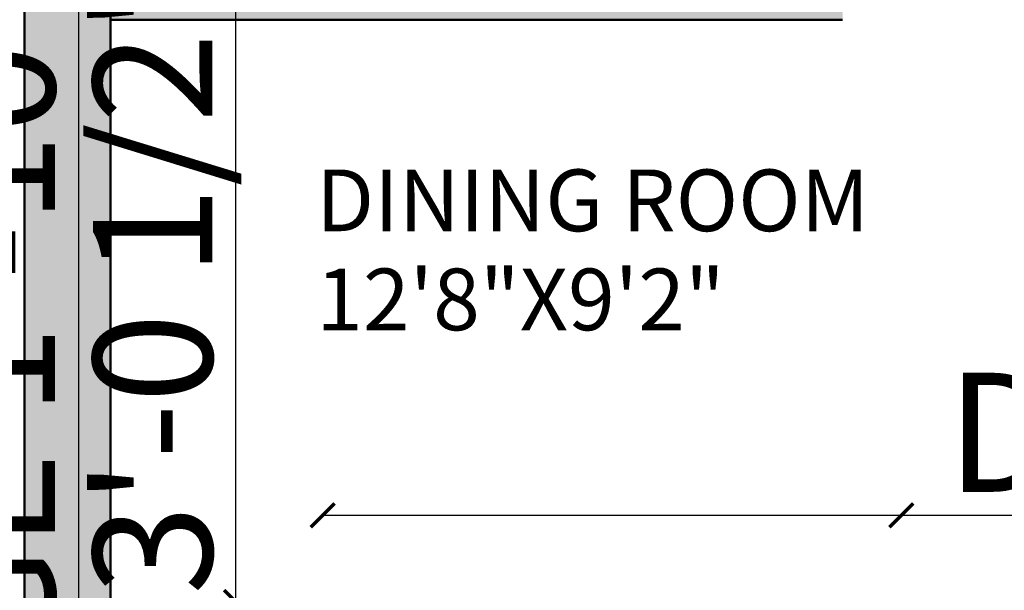
# Model space of a CAD drawing. Units: inches. Extents: x 2419 to 2878, y 1068 to 1713.
# Tile 7 of 20: x 2471 to 2574, y 1349 to 1409. Entities that reach past the tile are written whole.
import ezdxf

# ---------------------------------------------------------------- set-up
doc = ezdxf.new("R2010")
doc.units = ezdxf.units.IN
for name, color, linetype, lineweight in [('A-ANNO-DIMS', 2, 'Continuous', 18), ('A-AREA-IDEN', 7, 'Continuous', 18), ('A-FLOR-PRKG-PATT', 1, 'Continuous', 13), ('A-FURN-PATT', 254, 'Continuous', 13), ('A-WALL', 7, 'Continuous', 50)]:
    doc.layers.add(name, color=color, linetype=linetype, lineweight=lineweight)
doc.layers.add('A-FLOR-FIXT-PATT', color=254, linetype='Continuous', lineweight=13, true_color=0xd7ebd2)
doc.layers.add('A-WALL-PATT', color=18, linetype='Continuous', lineweight=13, true_color=0x000000)
doc.styles.get("Standard").update_dxf_attribs({"font": 'arial.ttf'})
doc.dimstyles.new('ISO-25', dxfattribs={"dimtxt": 12.5, "dimasz": 2.5, "dimexe": 1.25, "dimexo": 0.625, "dimtad": 1, "dimdec": 0, "dimlunit": 4, "dimtxsty": 'Standard', "dimblk": 'ARCHTICK', "dimcen": 2.5, "dimse1": 1, "dimse2": 1, "dimclrd": 4, "dimadec": 0, "dimazin": 0, "dimtfac": 1, "dimtdec": 0, "dimtmove": 0, "dimatfit": 3, "dimfxl": 1, "dimarcsym": 0})

# ---------------------------------------------------------------- blocks, each defined once
blk = doc.blocks.new('_ArchTick')
at = {"color": 0, "linetype": 'ByBlock', "const_width": 0.15}
blk.add_lwpolyline([(-0.5, -0.5), (0.5, 0.5)], dxfattribs=at)
blk = doc.blocks.new('*D26')
at = {"layer": 'A-ANNO-DIMS', "color": 4, "lineweight": -2, "transparency": 16777216}
for p, q in [((2502.77, 1356.79), (2563.46, 1356.79)), ((2563.46, 1356.79), (2733.72, 1356.79))]:
    blk.add_line(p, q, dxfattribs=at)
at = {"layer": 'Defpoints', "color": 0, "transparency": 16777216}
for p in [(2563.46, 1356.79), (2502.77, 1347.69), (2563.46, 1347.69)]:
    blk.add_point(p, dxfattribs=at)
at = {"layer": 'A-ANNO-DIMS', "color": 4, "lineweight": -2, "transparency": 16777216, "xscale": 2.5, "yscale": 2.5, "zscale": 2.5, "rotation": 180}
blk.add_blockref('_ArchTick', (2502.77, 1356.79), dxfattribs=at)
at = {"layer": 'A-ANNO-DIMS', "color": 4, "lineweight": -2, "transparency": 16777216, "xscale": 2.5, "yscale": 2.5, "zscale": 2.5}
blk.add_blockref('_ArchTick', (2563.46, 1356.79), dxfattribs=at)
at = {"layer": 'A-ANNO-DIMS', "color": 0, "transparency": 16777216, "insert": (2649.84, 1363.88), "char_height": 12.5, "attachment_point": 5}
blk.add_mtext('DINING SET 5\'-0 1/2"', dxfattribs=at)
blk = doc.blocks.new('*D27')
at = {"layer": 'A-ANNO-DIMS', "color": 4, "lineweight": -2, "transparency": 16777216}
for p, q in [((2493.67, 1347.69), (2493.67, 1413.78)), ((2493.67, 1311.01), (2493.67, 1347.69))]:
    blk.add_line(p, q, dxfattribs=at)
at = {"layer": 'Defpoints', "color": 0, "transparency": 16777216}
for p in [(2493.67, 1347.69), (2502.77, 1347.69), (2502.77, 1311.01)]:
    blk.add_point(p, dxfattribs=at)
at = {"layer": 'A-ANNO-DIMS', "color": 4, "lineweight": -2, "transparency": 16777216, "xscale": 2.5, "yscale": 2.5, "zscale": 2.5}
for p, rotation in [((2493.67, 1347.69), 90), ((2493.67, 1311.01), 270)]:
    blk.add_blockref('_ArchTick', p, dxfattribs=dict(at, rotation=rotation))
at = {"layer": 'A-ANNO-DIMS', "color": 0, "transparency": 16777216, "insert": (2486.57, 1381.99), "char_height": 12.5, "attachment_point": 5, "rotation": 90}
blk.add_mtext('3\'-0 1/2"', dxfattribs=at)
blk = doc.blocks.new('*D28')
at = {"layer": 'A-ANNO-DIMS', "color": 4, "lineweight": -2, "transparency": 16777216}
for p, q in [((2477.16, 1470.63), (2477.16, 1448.27)), ((2477.16, 1448.27), (2477.16, 1306.15))]:
    blk.add_line(p, q, dxfattribs=at)
at = {"layer": 'Defpoints', "color": 0, "transparency": 16777216}
for p in [(2480.51, 1470.63), (2477.16, 1448.27), (2480.51, 1448.27)]:
    blk.add_point(p, dxfattribs=at)
at = {"layer": 'A-ANNO-DIMS', "color": 4, "lineweight": -2, "transparency": 16777216, "xscale": 2.5, "yscale": 2.5, "zscale": 2.5}
for p, rotation in [((2477.16, 1470.63), 90), ((2477.16, 1448.27), 270)]:
    blk.add_blockref('_ArchTick', p, dxfattribs=dict(at, rotation=rotation))
at = {"layer": 'A-ANNO-DIMS', "color": 0, "transparency": 16777216, "insert": (2470.07, 1375.96), "char_height": 12.5, "attachment_point": 5, "rotation": 90}
blk.add_mtext('RANGE 1\'-10 1/2"', dxfattribs=at)
blk = doc.blocks.new('*D43')
at = {"layer": 'A-ANNO-DIMS', "color": 4, "lineweight": -2, "transparency": 16777216}
blk.add_line((2480.51, 1079.92), (2557.3, 1079.92), dxfattribs=at)
at = {"layer": 'Defpoints', "color": 0, "transparency": 16777216}
for p in [(2480.51, 1408.81), (2557.3, 1408.81), (2557.3, 1079.92)]:
    blk.add_point(p, dxfattribs=at)
at = {"layer": 'A-ANNO-DIMS', "color": 4, "lineweight": -2, "transparency": 16777216, "xscale": 2.5, "yscale": 2.5, "zscale": 2.5, "rotation": 180}
blk.add_blockref('_ArchTick', (2480.51, 1079.92), dxfattribs=at)
at = {"layer": 'A-ANNO-DIMS', "color": 4, "lineweight": -2, "transparency": 16777216, "xscale": 2.5, "yscale": 2.5, "zscale": 2.5}
blk.add_blockref('_ArchTick', (2557.3, 1079.92), dxfattribs=at)
at = {"layer": 'A-ANNO-DIMS', "color": 0, "transparency": 16777216, "insert": (2518.91, 1086.93), "char_height": 12.5, "attachment_point": 5}
blk.add_mtext('6\'-5"', dxfattribs=at)
blk = doc.blocks.new('*D44')
at = {"layer": 'A-ANNO-DIMS', "color": 4, "lineweight": -2, "transparency": 16777216}
for p, q in [((2557.3, 1079.92), (2585.82, 1079.92)), ((2585.82, 1079.92), (2652.14, 1079.92))]:
    blk.add_line(p, q, dxfattribs=at)
at = {"layer": 'Defpoints', "color": 0, "transparency": 16777216}
for p in [(2557.3, 1408.81), (2585.82, 1408.81), (2585.82, 1079.92)]:
    blk.add_point(p, dxfattribs=at)
at = {"layer": 'A-ANNO-DIMS', "color": 4, "lineweight": -2, "transparency": 16777216, "xscale": 2.5, "yscale": 2.5, "zscale": 2.5, "rotation": 180}
blk.add_blockref('_ArchTick', (2557.3, 1079.92), dxfattribs=at)
at = {"layer": 'A-ANNO-DIMS', "color": 4, "lineweight": -2, "transparency": 16777216, "xscale": 2.5, "yscale": 2.5, "zscale": 2.5}
blk.add_blockref('_ArchTick', (2585.82, 1079.92), dxfattribs=at)
at = {"layer": 'A-ANNO-DIMS', "color": 0, "transparency": 16777216, "insert": (2620.23, 1087.01), "char_height": 12.5, "attachment_point": 5}
blk.add_mtext('2\'-4 1/2"', dxfattribs=at)
blk = doc.blocks.new('*D47')
at = {"layer": 'A-ANNO-DIMS', "color": 4, "lineweight": -2, "transparency": 16777216}
for p, q in [((2444.31, 1376.56), (2444.31, 1357.98)), ((2444.31, 1357.98), (2444.31, 1293.05))]:
    blk.add_line(p, q, dxfattribs=at)
at = {"layer": 'Defpoints', "color": 0, "transparency": 16777216}
for p in [(2632.51, 1376.56), (2444.31, 1357.98), (2632.51, 1357.98)]:
    blk.add_point(p, dxfattribs=at)
at = {"layer": 'A-ANNO-DIMS', "color": 4, "lineweight": -2, "transparency": 16777216, "xscale": 2.5, "yscale": 2.5, "zscale": 2.5}
for p, rotation in [((2444.31, 1376.56), 90), ((2444.31, 1357.98), 270)]:
    blk.add_blockref('_ArchTick', p, dxfattribs=dict(at, rotation=rotation))
at = {"layer": 'A-ANNO-DIMS', "color": 0, "transparency": 16777216, "insert": (2437.23, 1324.26), "char_height": 12.5, "attachment_point": 5, "rotation": 90}
blk.add_mtext('1\'-6 1/2"', dxfattribs=at)
blk = doc.blocks.new('*D55')
at = {"layer": 'A-ANNO-DIMS', "color": 4, "lineweight": -2, "transparency": 16777216}
for p, q in [((2444.31, 1414.81), (2444.31, 1408.81)), ((2444.31, 1408.81), (2444.31, 1371.83))]:
    blk.add_line(p, q, dxfattribs=at)
at = {"layer": 'Defpoints', "color": 0, "transparency": 16777216}
for p in [(2480.51, 1414.81), (2444.31, 1408.81), (2480.51, 1408.81)]:
    blk.add_point(p, dxfattribs=at)
at = {"layer": 'A-ANNO-DIMS', "color": 4, "lineweight": -2, "transparency": 16777216, "xscale": 2.5, "yscale": 2.5, "zscale": 2.5}
for p, rotation in [((2444.31, 1414.81), 90), ((2444.31, 1408.81), 270)]:
    blk.add_blockref('_ArchTick', p, dxfattribs=dict(at, rotation=rotation))
at = {"layer": 'A-ANNO-DIMS', "color": 0, "transparency": 16777216, "insert": (2437.31, 1389.07), "char_height": 12.5, "attachment_point": 5, "rotation": 90}
blk.add_mtext('0\'-6"', dxfattribs=at)
blk = doc.blocks.new('*D56')
at = {"layer": 'A-ANNO-DIMS', "color": 4, "lineweight": -2, "transparency": 16777216}
for p, q in [((2480.51, 1079.92), (2503.97, 1079.92)), ((2503.97, 1079.92), (2578.61, 1079.92))]:
    blk.add_line(p, q, dxfattribs=at)
at = {"layer": 'Defpoints', "color": 0, "transparency": 16777216}
for p in [(2480.51, 1507.81), (2503.97, 1494.85), (2503.97, 1079.92)]:
    blk.add_point(p, dxfattribs=at)
at = {"layer": 'A-ANNO-DIMS', "color": 4, "lineweight": -2, "transparency": 16777216, "xscale": 2.5, "yscale": 2.5, "zscale": 2.5, "rotation": 180}
blk.add_blockref('_ArchTick', (2480.51, 1079.92), dxfattribs=at)
at = {"layer": 'A-ANNO-DIMS', "color": 4, "lineweight": -2, "transparency": 16777216, "xscale": 2.5, "yscale": 2.5, "zscale": 2.5}
blk.add_blockref('_ArchTick', (2503.97, 1079.92), dxfattribs=at)
at = {"layer": 'A-ANNO-DIMS', "color": 0, "transparency": 16777216, "insert": (2542.54, 1087.01), "char_height": 12.5, "attachment_point": 5}
blk.add_mtext('1\'-11 1/2"', dxfattribs=at)
blk = doc.blocks.new('*D59')
at = {"layer": 'A-ANNO-DIMS', "color": 4, "lineweight": -2, "transparency": 16777216}
blk.add_line((2480.51, 1079.92), (2589.51, 1079.92), dxfattribs=at)
at = {"layer": 'Defpoints', "color": 0, "transparency": 16777216}
for p in [(2480.51, 1414.81), (2589.51, 1414.81), (2589.51, 1079.92)]:
    blk.add_point(p, dxfattribs=at)
at = {"layer": 'A-ANNO-DIMS', "color": 4, "lineweight": -2, "transparency": 16777216, "xscale": 2.5, "yscale": 2.5, "zscale": 2.5, "rotation": 180}
blk.add_blockref('_ArchTick', (2480.51, 1079.92), dxfattribs=at)
at = {"layer": 'A-ANNO-DIMS', "color": 4, "lineweight": -2, "transparency": 16777216, "xscale": 2.5, "yscale": 2.5, "zscale": 2.5}
blk.add_blockref('_ArchTick', (2589.51, 1079.92), dxfattribs=at)
at = {"layer": 'A-ANNO-DIMS', "color": 0, "transparency": 16777216, "insert": (2535.01, 1086.93), "char_height": 12.5, "attachment_point": 5}
blk.add_mtext('9\'-1"', dxfattribs=at)

msp = doc.modelspace()

# ---------------------------------------------------------------- hatches: boundary and pattern name
at = {"layer": 'A-FLOR-FIXT-PATT'}
h = msp.add_hatch(color=256, dxfattribs=at)
h.dxf.hatch_style = 1
h.paths.add_polyline_path([(2771.51, 1458.39), (2763.51, 1458.39), (2763.51, 1437.39), (2771.51, 1437.39)])
h.paths.add_polyline_path([(2770.51, 1456.39, 0.5), (2769.51, 1457.39), (2765.51, 1457.39, 0.5), (2764.51, 1456.39), (2764.51, 1439.39, 0.5), (2765.51, 1438.39), (2769.51, 1438.39, 0.5), (2770.51, 1439.39)], flags=16)
h.paths.add_polyline_path([(2706.38, 1408.81), (2685.38, 1408.81), (2685.38, 1400.81), (2706.38, 1400.81)])
h.paths.add_polyline_path([(2704.38, 1401.81, 0.5), (2705.38, 1402.81), (2705.38, 1406.81, 0.5), (2704.38, 1407.81), (2687.38, 1407.81, 0.5), (2686.38, 1406.81), (2686.38, 1402.81, 0.5), (2687.38, 1401.81)], flags=16)
h.paths.add_polyline_path([(2574.48, 1207.45), (2633.94, 1207.45), (2633.94, 1217.37), (2574.48, 1217.37)], flags=9)
h.paths.add_polyline_path([(2574.45, 1217.83), (2610.47, 1217.83), (2610.47, 1227.88), (2574.45, 1227.88)], flags=9)
h.paths.add_polyline_path([(2672.43, 1304.02), (2718.62, 1304.02), (2718.62, 1313.94), (2672.43, 1313.94)], flags=9)
h.paths.add_polyline_path([(2672.4, 1314.4), (2750.13, 1314.4), (2750.13, 1324.45), (2672.4, 1324.45)], flags=9)
h.paths.add_polyline_path([(2500.43, 1374.44), (2544.8, 1374.44), (2544.8, 1384.36), (2500.43, 1384.36)], flags=9)
h.paths.add_polyline_path([(2500.41, 1384.82), (2566.08, 1384.82), (2566.08, 1394.87), (2500.41, 1394.87)], flags=9)
h.paths.add_polyline_path([(2738.93, 1376.75), (2778.27, 1376.75), (2778.27, 1386.67), (2738.93, 1386.67)], flags=9)
h.paths.add_polyline_path([(2659.12, 1357.8), (2703.49, 1357.8), (2703.49, 1367.72), (2659.12, 1367.72)], flags=9)
h.paths.add_polyline_path([(2659.1, 1368.18), (2694.11, 1368.18), (2694.11, 1378.23), (2659.1, 1378.23)], flags=9)
h.paths.add_polyline_path([(2730.12, 1466.07), (2769.46, 1466.07), (2769.46, 1475.99), (2730.12, 1475.99)], flags=9)
h.paths.add_polyline_path([(2730.1, 1476.45), (2765.12, 1476.45), (2765.12, 1486.5), (2730.1, 1486.5)], flags=9)
h.paths.add_polyline_path([(2730.38, 1518.65), (2761.48, 1518.65), (2761.48, 1528.57), (2730.38, 1528.57)], flags=9)
h.paths.add_polyline_path([(2730.36, 1529.03), (2780.96, 1529.03), (2780.96, 1539.07), (2730.36, 1539.07)], flags=9)
h.paths.add_polyline_path([(2629.32, 1455.19), (2688.78, 1455.19), (2688.78, 1465.11), (2629.32, 1465.11)], flags=9)
h.paths.add_polyline_path([(2629.3, 1465.57), (2681.9, 1465.57), (2681.9, 1475.62), (2629.3, 1475.62)], flags=9)
h.paths.add_polyline_path([(2513.23, 1456.48), (2562.63, 1456.48), (2562.63, 1466.4), (2513.23, 1466.4)], flags=9)
h.paths.add_polyline_path([(2513.21, 1466.86), (2556.26, 1466.86), (2556.26, 1476.91), (2513.21, 1476.91)], flags=9)
h.paths.add_polyline_path([(2488.87, 1521.54), (2519.97, 1521.54), (2519.97, 1531.46), (2488.87, 1531.46)], flags=9)
h.paths.add_polyline_path([(2536.55, 1543.51), (2580.92, 1543.51), (2580.92, 1553.43), (2536.55, 1553.43)], flags=9)
h.paths.add_polyline_path([(2536.56, 1553.92), (2573.53, 1553.92), (2573.53, 1563.8), (2536.56, 1563.8)], flags=9)
at = {"layer": 'A-FLOR-PRKG-PATT'}
h = msp.add_hatch(color=256, dxfattribs=at)
h.dxf.hatch_style = 1
edge = h.paths.add_edge_path()
edge.add_ellipse((2561.37, 1279.45), major_axis=(3.99, 0), ratio=0.842304, start_angle=0.6466, end_angle=90)
edge.add_line((2561.37, 1282.81), (2511.57, 1282.81))
edge.add_ellipse((2511.57, 1279.45), major_axis=(3.99, 0), ratio=0.842304, start_angle=90, end_angle=179.3534)
edge.add_ellipse((10560.89, 1188.62), major_axis=(-8054.03, 0), ratio=0.8423039, start_angle=-0.646554, end_angle=-0.628237)
edge.add_ellipse((2509.23, 1276.91), major_axis=(1.69, 0), ratio=0.842304, start_angle=179.3718, end_angle=248.4648)
edge.add_ellipse((10560.33, 1188.62), major_axis=(8052.29, 0), ratio=0.8423039, start_angle=179.353446, end_angle=179.381357, ccw=False)
edge.add_ellipse((2511.01, 1279.45), major_axis=(2.25, 0), ratio=0.842304, start_angle=90, end_angle=179.3534, ccw=False)
edge.add_line((2511.01, 1281.35), (2561.94, 1281.35))
edge.add_ellipse((2561.94, 1279.45), major_axis=(-2.25, 0), ratio=0.842304, start_angle=180.6466, end_angle=270, ccw=False)
edge.add_ellipse((-5487.38, 1188.62), major_axis=(8052.29, 0), ratio=0.8423039, start_angle=0.528271, end_angle=0.646554, ccw=False)
edge.add_ellipse((2563.71, 1276.91), major_axis=(-1.69, 0), ratio=0.842304, start_angle=111.5352, end_angle=180.6282)
edge.add_ellipse((-5487.95, 1188.62), major_axis=(-8054.03, 0), ratio=0.8423039, start_angle=180.628237, end_angle=180.646554)
edge = h.paths.add_edge_path()
edge.add_ellipse((2564.91, 1261.91), major_axis=(-1.12, 0), ratio=0.842304, start_angle=180, end_angle=270)
edge.add_line((2564.91, 1262.86), (2564.43, 1262.86))
edge.add_ellipse((-5487.38, 1188.62), major_axis=(8052.29, 0), ratio=0.8423039, start_angle=0.383867, end_angle=0.528271, ccw=False)
edge.add_line((2564.65, 1242.56), (2564.91, 1242.56))
edge.add_ellipse((2564.91, 1243.51), major_axis=(-1.12, 0), ratio=0.842304, start_angle=90, end_angle=180)
edge.add_line((2566.03, 1243.51), (2566.03, 1261.91))
edge = h.paths.add_edge_path()
edge.add_ellipse((2564.91, 1174.99), major_axis=(1.12, 0), ratio=0.842304, start_angle=0, end_angle=90)
edge.add_line((2564.91, 1175.94), (2564.89, 1175.94))
edge.add_ellipse((-5487.38, 1188.62), major_axis=(8052.29, 0), ratio=0.8423039, start_angle=-0.134987, end_angle=-0.090229, ccw=False)
edge.add_ellipse((2163.34, 1170.91), major_axis=(401.54, 0), ratio=0.842304, start_angle=-2.18, end_angle=-0.1356, ccw=False)
edge.add_line((2564.47, 1155.64), (2564.91, 1155.64))
edge.add_ellipse((2564.91, 1156.59), major_axis=(-1.12, 0), ratio=0.842304, start_angle=90, end_angle=180)
edge.add_line((2566.03, 1156.59), (2566.03, 1174.99))
h.paths.add_polyline_path([(2574.48, 1207.45), (2633.94, 1207.45), (2633.94, 1217.37), (2574.48, 1217.37)], flags=9)
h.paths.add_polyline_path([(2574.45, 1217.83), (2610.47, 1217.83), (2610.47, 1227.88), (2574.45, 1227.88)], flags=9)
h.paths.add_polyline_path([(2672.43, 1304.02), (2718.62, 1304.02), (2718.62, 1313.94), (2672.43, 1313.94)], flags=9)
h.paths.add_polyline_path([(2672.4, 1314.4), (2750.13, 1314.4), (2750.13, 1324.45), (2672.4, 1324.45)], flags=9)
h.paths.add_polyline_path([(2500.43, 1374.44), (2544.8, 1374.44), (2544.8, 1384.36), (2500.43, 1384.36)], flags=9)
h.paths.add_polyline_path([(2500.41, 1384.82), (2566.08, 1384.82), (2566.08, 1394.87), (2500.41, 1394.87)], flags=9)
h.paths.add_polyline_path([(2738.93, 1376.75), (2778.27, 1376.75), (2778.27, 1386.67), (2738.93, 1386.67)], flags=9)
h.paths.add_polyline_path([(2659.12, 1357.8), (2703.49, 1357.8), (2703.49, 1367.72), (2659.12, 1367.72)], flags=9)
h.paths.add_polyline_path([(2659.1, 1368.18), (2694.11, 1368.18), (2694.11, 1378.23), (2659.1, 1378.23)], flags=9)
h.paths.add_polyline_path([(2730.12, 1466.07), (2769.46, 1466.07), (2769.46, 1475.99), (2730.12, 1475.99)], flags=9)
h.paths.add_polyline_path([(2730.1, 1476.45), (2765.12, 1476.45), (2765.12, 1486.5), (2730.1, 1486.5)], flags=9)
h.paths.add_polyline_path([(2730.38, 1518.65), (2761.48, 1518.65), (2761.48, 1528.57), (2730.38, 1528.57)], flags=9)
h.paths.add_polyline_path([(2730.36, 1529.03), (2780.96, 1529.03), (2780.96, 1539.07), (2730.36, 1539.07)], flags=9)
h.paths.add_polyline_path([(2629.32, 1455.19), (2688.78, 1455.19), (2688.78, 1465.11), (2629.32, 1465.11)], flags=9)
h.paths.add_polyline_path([(2629.3, 1465.57), (2681.9, 1465.57), (2681.9, 1475.62), (2629.3, 1475.62)], flags=9)
h.paths.add_polyline_path([(2513.23, 1456.48), (2562.63, 1456.48), (2562.63, 1466.4), (2513.23, 1466.4)], flags=9)
h.paths.add_polyline_path([(2513.21, 1466.86), (2556.26, 1466.86), (2556.26, 1476.91), (2513.21, 1476.91)], flags=9)
h.paths.add_polyline_path([(2488.87, 1521.54), (2519.97, 1521.54), (2519.97, 1531.46), (2488.87, 1531.46)], flags=9)
h.paths.add_polyline_path([(2536.55, 1543.51), (2580.92, 1543.51), (2580.92, 1553.43), (2536.55, 1553.43)], flags=9)
h.paths.add_polyline_path([(2536.56, 1553.92), (2573.53, 1553.92), (2573.53, 1563.8), (2536.56, 1563.8)], flags=9)
at = {"layer": 'A-FURN-PATT'}
h = msp.add_hatch(color=256, dxfattribs=at)
h.dxf.hatch_style = 1
h.paths.add_polyline_path([(2710.17, 1562.64), (2707.17, 1559.64), (2709.17, 1559.64, -0.414214), (2710.17, 1560.64)])
h.paths.add_polyline_path([(2711.17, 1559.64, 1), (2709.17, 1559.64, 1)])
h.paths.add_polyline_path([(2710.17, 1562.64), (2710.17, 1560.64, -0.414214), (2711.17, 1559.64), (2713.17, 1559.64)])
h.paths.add_polyline_path([(2713.17, 1559.64), (2711.17, 1559.64, -0.414214), (2710.17, 1558.64), (2710.17, 1556.64)])
h.paths.add_polyline_path([(2710.17, 1558.64, -0.414214), (2709.17, 1559.64), (2707.17, 1559.64), (2710.17, 1556.64)])
h.paths.add_polyline_path([(2613.13, 1558.89, 1), (2611.13, 1558.89, 1)])
h.paths.add_polyline_path([(2612.13, 1561.89), (2612.13, 1559.89, -0.414214), (2613.13, 1558.89), (2615.13, 1558.89)])
h.paths.add_polyline_path([(2612.13, 1559.89), (2612.13, 1561.89), (2609.13, 1558.89), (2611.13, 1558.89, -0.414214)])
h.paths.add_polyline_path([(2612.13, 1557.89, -0.414214), (2611.13, 1558.89), (2609.13, 1558.89), (2612.13, 1555.89)])
h.paths.add_polyline_path([(2574.48, 1207.45), (2633.94, 1207.45), (2633.94, 1217.37), (2574.48, 1217.37)], flags=9)
h.paths.add_polyline_path([(2574.45, 1217.83), (2610.47, 1217.83), (2610.47, 1227.88), (2574.45, 1227.88)], flags=9)
h.paths.add_polyline_path([(2672.43, 1304.02), (2718.62, 1304.02), (2718.62, 1313.94), (2672.43, 1313.94)], flags=9)
h.paths.add_polyline_path([(2672.4, 1314.4), (2750.13, 1314.4), (2750.13, 1324.45), (2672.4, 1324.45)], flags=9)
h.paths.add_polyline_path([(2500.43, 1374.44), (2544.8, 1374.44), (2544.8, 1384.36), (2500.43, 1384.36)], flags=9)
h.paths.add_polyline_path([(2500.41, 1384.82), (2566.08, 1384.82), (2566.08, 1394.87), (2500.41, 1394.87)], flags=9)
h.paths.add_polyline_path([(2738.93, 1376.75), (2778.27, 1376.75), (2778.27, 1386.67), (2738.93, 1386.67)], flags=9)
h.paths.add_polyline_path([(2659.12, 1357.8), (2703.49, 1357.8), (2703.49, 1367.72), (2659.12, 1367.72)], flags=9)
h.paths.add_polyline_path([(2659.1, 1368.18), (2694.11, 1368.18), (2694.11, 1378.23), (2659.1, 1378.23)], flags=9)
h.paths.add_polyline_path([(2730.12, 1466.07), (2769.46, 1466.07), (2769.46, 1475.99), (2730.12, 1475.99)], flags=9)
h.paths.add_polyline_path([(2730.1, 1476.45), (2765.12, 1476.45), (2765.12, 1486.5), (2730.1, 1486.5)], flags=9)
h.paths.add_polyline_path([(2730.38, 1518.65), (2761.48, 1518.65), (2761.48, 1528.57), (2730.38, 1528.57)], flags=9)
h.paths.add_polyline_path([(2730.36, 1529.03), (2780.96, 1529.03), (2780.96, 1539.07), (2730.36, 1539.07)], flags=9)
h.paths.add_polyline_path([(2629.32, 1455.19), (2688.78, 1455.19), (2688.78, 1465.11), (2629.32, 1465.11)], flags=9)
h.paths.add_polyline_path([(2629.3, 1465.57), (2681.9, 1465.57), (2681.9, 1475.62), (2629.3, 1475.62)], flags=9)
h.paths.add_polyline_path([(2513.23, 1456.48), (2562.63, 1456.48), (2562.63, 1466.4), (2513.23, 1466.4)], flags=9)
h.paths.add_polyline_path([(2513.21, 1466.86), (2556.26, 1466.86), (2556.26, 1476.91), (2513.21, 1476.91)], flags=9)
h.paths.add_polyline_path([(2488.87, 1521.54), (2519.97, 1521.54), (2519.97, 1531.46), (2488.87, 1531.46)], flags=9)
h.paths.add_polyline_path([(2536.55, 1543.51), (2580.92, 1543.51), (2580.92, 1553.43), (2536.55, 1553.43)], flags=9)
h.paths.add_polyline_path([(2536.56, 1553.92), (2573.53, 1553.92), (2573.53, 1563.8), (2536.56, 1563.8)], flags=9)
at = {"layer": 'A-WALL-PATT'}
h = msp.add_hatch(color=256, dxfattribs=at)
h.dxf.hatch_style = 1
h.paths.add_polyline_path([(2780.51, 1577.81), (2471.51, 1577.81), (2471.51, 1121.81), (2780.51, 1121.81)])
h.paths.add_polyline_path([(2480.51, 1568.81), (2771.51, 1568.81), (2771.51, 1130.81), (2480.51, 1130.81)], flags=16)
h.paths.add_polyline_path([(2528.51, 1568.81), (2528.51, 1512.81), (2594.51, 1512.81), (2594.51, 1414.81), (2596.57, 1414.81), (2596.57, 1441.61), (2597.82, 1441.61), (2597.82, 1441.58, -0.384016), (2625.03, 1414.81), (2725.51, 1414.81), (2725.51, 1567.55), (2728.3, 1567.55), (2746.89, 1567.55), (2746.89, 1566.73), (2746.87, 1566.73, -0.367216), (2730.51, 1549.09), (2730.51, 1512.81), (2750.85, 1512.81), (2750.85, 1510.03, -0.401453), (2733.08, 1491.46), (2733.08, 1491.44), (2732.27, 1491.44), (2732.27, 1507.81), (2730.51, 1507.81), (2730.51, 1408.81), (2736.51, 1408.81), (2736.51, 1349.81), (2632.51, 1349.81), (2632.51, 1408.81), (2528.51, 1408.81), (2528.51, 1414.81), (2503.97, 1414.81), (2503.97, 1494.85), (2558.38, 1494.85), (2558.38, 1507.81), (2529.96, 1507.81, -0.414214), (2530.82, 1506.96), (2530.82, 1497.26, -0.414214), (2529.96, 1496.4), (2514.56, 1496.4, -0.414214), (2513.7, 1497.26), (2513.7, 1506.96, -0.414214), (2514.56, 1507.81), (2528.51, 1507.81), (2528.51, 1512.81), (2480.51, 1512.81)], flags=0)
h.paths.add_polyline_path([(2516.26, 1507.81), (2528.26, 1507.81), (2528.26, 1505.81), (2523.42, 1505.81), (2524.07, 1504.67), (2529.39, 1504.67, -0.414214), (2529.96, 1504.1), (2529.96, 1497.83, -0.414214), (2529.39, 1497.26), (2515.13, 1497.26, -0.414214), (2514.56, 1497.83), (2514.56, 1504.1, -0.414214), (2515.13, 1504.67), (2520.69, 1504.67), (2521.34, 1505.81), (2516.26, 1505.81)], flags=0)
h.paths.add_polyline_path([(2522.02, 1505.53), (2522.82, 1507.32, -0.65506), (2522.25, 1506.06), (2522.19, 1505.93), (2522.43, 1505.53)], flags=0)
h.paths.add_polyline_path([(2522.83, 1500.97, -1), (2521.69, 1500.97, -1)], flags=0)
h.paths.add_polyline_path([(2522.55, 1500.97, -1), (2521.98, 1500.97, -1)], flags=0)
h.paths.add_polyline_path([(2482.01, 1470.63), (2499.89, 1470.63), (2499.89, 1448.27), (2482.01, 1448.27), (2482.01, 1452.74), (2481.26, 1452.74), (2481.26, 1449.76), (2480.51, 1449.76), (2480.51, 1469.14), (2481.26, 1469.14), (2481.26, 1466.16), (2482.01, 1466.16)], flags=0)
h.paths.add_polyline_path([(2488.71, 1466.16, -1), (2484.24, 1466.16, -1)], flags=0)
h.paths.add_polyline_path([(2496.17, 1466.16, -1), (2490.2, 1466.16, -1)], flags=0)
h.paths.add_polyline_path([(2487.97, 1466.16, -1), (2484.99, 1466.16, -1)], flags=0)
h.paths.add_polyline_path([(2495.42, 1466.16, -1), (2490.95, 1466.16, -1)], flags=0)
h.paths.add_polyline_path([(2487.22, 1466.16, -1), (2485.73, 1466.16, -1)], flags=0)
h.paths.add_polyline_path([(2494.68, 1466.16, -1), (2491.69, 1466.16, -1)], flags=0)
h.paths.add_polyline_path([(2499.11, 1468, -1), (2497.98, 1468, -1)], flags=0)
h.paths.add_polyline_path([(2493.93, 1466.16, -1), (2492.44, 1466.16, -1)], flags=0)
h.paths.add_polyline_path([(2499.37, 1463.71, -1), (2498.17, 1463.71, -1)], flags=0)
h.paths.add_polyline_path([(2484.24, 1461.69), (2496.17, 1461.69), (2496.17, 1457.22), (2484.24, 1457.22)], flags=0)
h.paths.add_polyline_path([(2484.99, 1460.94), (2495.42, 1460.94), (2495.42, 1457.96), (2484.99, 1457.96)], flags=0)
h.paths.add_polyline_path([(2586.88, 1510.03), (2587.69, 1510.03), (2587.69, 1491.44), (2586.88, 1491.44)], flags=0)
h.paths.add_polyline_path([(2499.26, 1459.41, -1), (2498.2, 1459.41, -1)], flags=0)
h.paths.add_polyline_path([(2489.46, 1452.74, -1), (2483.5, 1452.74, -1)], flags=0)
h.paths.add_polyline_path([(2557.3, 1408.81), (2557.3, 1413.09, -0.401453), (2584.57, 1441.58), (2584.57, 1441.61), (2585.82, 1441.61), (2585.82, 1413.09), (2585.82, 1408.81)], flags=0)
h.paths.add_polyline_path([(2488.71, 1452.74, -1), (2484.24, 1452.74, -1)], flags=0)
h.paths.add_polyline_path([(2495.42, 1452.74, -1), (2490.95, 1452.74, -1)], flags=0)
h.paths.add_polyline_path([(2487.97, 1452.74, -1), (2484.99, 1452.74, -1)], flags=0)
h.paths.add_polyline_path([(2494.68, 1452.74, -1), (2491.69, 1452.74, -1)], flags=0)
h.paths.add_polyline_path([(2487.22, 1452.74, -1), (2485.73, 1452.74, -1)], flags=0)
h.paths.add_polyline_path([(2499.18, 1454.44, -1), (2497.9, 1454.44, -1)], flags=0)
h.paths.add_polyline_path([(2493.93, 1452.74, -1), (2492.44, 1452.74, -1)], flags=0)
h.paths.add_polyline_path([(2499.3, 1450.64, -1), (2497.79, 1450.64, -1)], flags=0)
h.paths.add_polyline_path([(2619.13, 1558.89, -1), (2605.13, 1558.89, -1)], flags=0)
h.paths.add_polyline_path([(2609.13, 1558.89), (2612.13, 1561.89), (2615.13, 1558.89), (2612.13, 1555.89)], flags=0)
h.paths.add_polyline_path([(2611.13, 1558.89, -1), (2613.13, 1558.89, -1)], flags=0)
h.paths.add_polyline_path([(2633.68, 1568.81), (2693.68, 1568.81), (2693.68, 1488.81), (2633.68, 1488.81)], flags=0)
h.paths.add_polyline_path([(2641.68, 1554.41), (2641.68, 1567.61), (2662.48, 1567.61), (2662.48, 1554.41), (2664.88, 1554.41), (2664.88, 1567.61), (2685.68, 1567.61), (2685.68, 1552.41), (2680.48, 1552.41), (2693.68, 1539.21), (2678.48, 1539.21), (2678.48, 1554.41)], flags=0)
h.paths.add_polyline_path([(2637.51, 1408.81), (2731.51, 1408.81), (2731.51, 1354.81), (2637.51, 1354.81), (2637.51, 1357.98), (2635.3, 1357.98), (2635.3, 1358.79), (2637.51, 1358.79)], flags=0)
h.paths.add_polyline_path([(2717.17, 1559.64, -1), (2703.17, 1559.64, -1)], flags=0)
h.paths.add_polyline_path([(2707.17, 1559.64), (2710.17, 1562.64), (2713.17, 1559.64), (2710.17, 1556.64)], flags=0)
h.paths.add_polyline_path([(2709.17, 1559.64, -1), (2711.17, 1559.64, -1)], flags=0)
h.paths.add_polyline_path([(2685.38, 1408.81), (2706.38, 1408.81), (2706.38, 1400.81), (2699.88, 1400.81), (2701.88, 1394.81, -0.501323), (2696.92, 1375.95, -0.132891), (2694.83, 1375.95, -0.501317), (2689.88, 1394.81), (2691.88, 1400.81), (2688.88, 1400.81), (2688.88, 1399.31), (2685.88, 1399.31), (2685.88, 1400.31), (2687.88, 1400.31), (2687.88, 1400.81), (2685.38, 1400.81)], flags=0)
h.paths.add_polyline_path([(2687.38, 1407.81), (2704.38, 1407.81, -0.5), (2705.38, 1406.81), (2705.38, 1402.81, -0.5), (2704.38, 1401.81), (2687.38, 1401.81, -0.5), (2686.38, 1402.81), (2686.38, 1406.81, -0.5)], flags=0)
h.paths.add_polyline_path([(2639.51, 1205.81), (2634.51, 1205.81), (2634.51, 1293.81), (2637.51, 1293.81), (2639.51, 1293.81)], flags=0)
h.paths.add_polyline_path([(2691.88, 1394.81), (2699.88, 1394.81, -0.48008), (2697.52, 1377.29, -0.215004), (2694.23, 1377.29, -0.48008)], flags=0)
h.paths.add_polyline_path([(2757.51, 1453.89), (2763.51, 1451.89), (2763.51, 1454.89), (2762.01, 1454.89), (2762.01, 1457.89), (2763.01, 1457.89), (2763.01, 1455.89), (2763.51, 1455.89), (2763.51, 1458.39), (2771.51, 1458.39), (2771.51, 1437.39), (2763.51, 1437.39), (2763.51, 1443.89), (2757.51, 1441.89, -0.501323), (2738.65, 1446.85, -0.132891), (2738.65, 1448.94, -0.501317)], flags=0)
h.paths.add_polyline_path([(2739.99, 1449.54, -0.48008), (2757.51, 1451.89), (2757.51, 1443.89, -0.48008), (2739.99, 1446.25, -0.215004)], flags=0)
h.paths.add_polyline_path([(2765.51, 1457.39), (2769.51, 1457.39, -0.5), (2770.51, 1456.39), (2770.51, 1439.39, -0.5), (2769.51, 1438.39), (2765.51, 1438.39, -0.5), (2764.51, 1439.39), (2764.51, 1456.39, -0.5)], flags=0)
h = msp.add_hatch(color=256, dxfattribs=at)
h.dxf.hatch_style = 1
h.paths.add_polyline_path([(2771.51, 1354.81), (2736.51, 1354.81), (2736.51, 1408.81), (2771.51, 1408.81), (2771.51, 1414.81), (2625.03, 1414.81, -0.015108), (2625.09, 1413.09), (2625.09, 1408.81), (2632.51, 1408.81), (2632.51, 1376.56), (2635.3, 1376.56, -0.029838), (2637.51, 1376.43), (2637.51, 1408.81), (2731.51, 1408.81), (2731.51, 1354.81), (2637.51, 1354.81), (2637.51, 1357.98), (2635.3, 1357.98), (2632.51, 1357.98), (2632.51, 1349.81), (2771.51, 1349.81)])
h.paths.add_polyline_path([(2639.51, 1298.81), (2637.51, 1298.81), (2480.51, 1298.81), (2480.51, 1293.81), (2637.51, 1293.81), (2639.51, 1293.81)])
h.paths.add_polyline_path([(2639.51, 1293.81), (2637.51, 1293.81), (2634.51, 1293.81), (2634.51, 1244.65), (2638.79, 1244.65, -0.006332), (2639.51, 1244.64)])
h.paths.add_polyline_path([(2639.51, 1205.81), (2771.51, 1205.81), (2771.51, 1210.81), (2639.51, 1210.81), (2639.51, 1216.13), (2638.79, 1216.13), (2634.51, 1216.13), (2634.51, 1130.81), (2639.51, 1130.81)])
h.paths.add_polyline_path([(2596.57, 1413.09), (2596.57, 1414.81), (2585.82, 1414.81), (2585.82, 1413.09), (2585.82, 1408.81), (2596.57, 1408.81)])
h.paths.add_polyline_path([(2557.3, 1413.09, -0.015108), (2557.35, 1414.81), (2480.51, 1414.81), (2480.51, 1408.81), (2557.3, 1408.81)])
h.paths.add_polyline_path([(2574.48, 1207.45), (2633.94, 1207.45), (2633.94, 1217.37), (2574.48, 1217.37)], flags=9)
h.paths.add_polyline_path([(2574.45, 1217.83), (2610.47, 1217.83), (2610.47, 1227.88), (2574.45, 1227.88)], flags=9)
h.paths.add_polyline_path([(2672.43, 1304.02), (2718.62, 1304.02), (2718.62, 1313.94), (2672.43, 1313.94)], flags=9)
h.paths.add_polyline_path([(2672.4, 1314.4), (2750.13, 1314.4), (2750.13, 1324.45), (2672.4, 1324.45)], flags=9)
h.paths.add_polyline_path([(2500.43, 1374.44), (2544.8, 1374.44), (2544.8, 1384.36), (2500.43, 1384.36)], flags=9)
h.paths.add_polyline_path([(2500.41, 1384.82), (2566.08, 1384.82), (2566.08, 1394.87), (2500.41, 1394.87)], flags=9)
h.paths.add_polyline_path([(2738.93, 1376.75), (2778.27, 1376.75), (2778.27, 1386.67), (2738.93, 1386.67)], flags=9)
h.paths.add_polyline_path([(2659.12, 1357.8), (2703.49, 1357.8), (2703.49, 1367.72), (2659.12, 1367.72)], flags=25)
h.paths.add_polyline_path([(2659.1, 1368.18), (2694.11, 1368.18), (2694.11, 1378.23), (2659.1, 1378.23)], flags=25)
h.paths.add_polyline_path([(2730.12, 1466.07), (2769.46, 1466.07), (2769.46, 1475.99), (2730.12, 1475.99)], flags=9)
h.paths.add_polyline_path([(2730.1, 1476.45), (2765.12, 1476.45), (2765.12, 1486.5), (2730.1, 1486.5)], flags=9)
h.paths.add_polyline_path([(2730.38, 1518.65), (2761.48, 1518.65), (2761.48, 1528.57), (2730.38, 1528.57)], flags=9)
h.paths.add_polyline_path([(2730.36, 1529.03), (2780.96, 1529.03), (2780.96, 1539.07), (2730.36, 1539.07)], flags=9)
h.paths.add_polyline_path([(2629.32, 1455.19), (2688.78, 1455.19), (2688.78, 1465.11), (2629.32, 1465.11)], flags=9)
h.paths.add_polyline_path([(2629.3, 1465.57), (2681.9, 1465.57), (2681.9, 1475.62), (2629.3, 1475.62)], flags=9)
h.paths.add_polyline_path([(2513.23, 1456.48), (2562.63, 1456.48), (2562.63, 1466.4), (2513.23, 1466.4)], flags=9)
h.paths.add_polyline_path([(2513.21, 1466.86), (2556.26, 1466.86), (2556.26, 1476.91), (2513.21, 1476.91)], flags=9)
h.paths.add_polyline_path([(2488.87, 1521.54), (2519.97, 1521.54), (2519.97, 1531.46), (2488.87, 1531.46)], flags=9)
h.paths.add_polyline_path([(2536.55, 1543.51), (2580.92, 1543.51), (2580.92, 1553.43), (2536.55, 1553.43)], flags=9)
h.paths.add_polyline_path([(2536.56, 1553.92), (2573.53, 1553.92), (2573.53, 1563.8), (2536.56, 1563.8)], flags=9)

# ---------------------------------------------------------------- linework, layer by layer
at = {"layer": 'A-WALL'}
for p, q in [((2480.51, 1130.81), (2480.51, 1568.81)), ((2480.51, 1408.81), (2557.3, 1408.81)), ((2480.51, 1408.81), (2557.3, 1408.81))]:
    msp.add_line(p, q, dxfattribs=at)
msp.add_lwpolyline([(2471.51, 1577.81), (2780.51, 1577.81), (2780.51, 1121.81), (2471.51, 1121.81)], close=True, dxfattribs=at)

# ---------------------------------------------------------------- texts
at = {"layer": 'A-AREA-IDEN'}
for s, height, p in [('DINING ROOM', 6.4753, (2502.09, 1386.61)), ('12\'8"X9\'2"', 6.475, (2502.09, 1376.21))]:
    msp.add_text(s, height=height, dxfattribs=at).set_placement(p)

# ---------------------------------------------------------------- dimensions: what is measured, and where the dimension line sits
at = {"layer": 'A-ANNO-DIMS'}
for base, p1, p2, picture, middle in [((2503.97, 1079.92), (2480.51, 1507.81), (2503.97, 1494.85), '*D56', (2542.54, 1087.01)), ((2589.51, 1079.92), (2480.51, 1414.81), (2589.51, 1414.81), '*D59', (2535.01, 1086.93)), ((2557.3, 1079.92), (2480.51, 1408.81), (2557.3, 1408.81), '*D43', (2518.91, 1086.93)), ((2585.82, 1079.92), (2557.3, 1408.81), (2585.82, 1408.81), '*D44', (2620.23, 1087.01))]:
    dim = msp.add_linear_dim(base=base, p1=p1, p2=p2, dimstyle='ISO-25', override={"dimdec": 1, "dimlfac": 1, "dimrnd": 0, "dimzin": 1, "dimdsep": 46, "dimlunit": 4, "dimfrac": 2}, dxfattribs=at)
    dim.commit()
    dim.dimension.update_dxf_attribs({"geometry": picture, "text_midpoint": middle})
dim = msp.add_linear_dim(base=(2477.16, 1448.27), p1=(2480.51, 1470.63), p2=(2480.51, 1448.27), angle=270, text='RANGE <>', dimstyle='ISO-25', override={"dimdec": 1, "dimlfac": 1, "dimrnd": 0, "dimzin": 1, "dimdsep": 46, "dimlunit": 4, "dimfrac": 2}, dxfattribs=at)
dim.commit()
dim.dimension.update_dxf_attribs({"geometry": '*D28', "text_midpoint": (2470.07, 1375.96)})
for base, p1, p2, picture, middle in [((2444.31, 1408.81), (2480.51, 1414.81), (2480.51, 1408.81), '*D55', (2437.31, 1389.07)), ((2493.67, 1347.69), (2502.77, 1311.01), (2502.77, 1347.69), '*D27', (2486.57, 1381.99)), ((2444.31, 1357.98), (2632.51, 1376.56), (2632.51, 1357.98), '*D47', (2437.23, 1324.26))]:
    dim = msp.add_linear_dim(base=base, p1=p1, p2=p2, angle=90, dimstyle='ISO-25', override={"dimdec": 1, "dimlfac": 1, "dimrnd": 0, "dimzin": 1, "dimdsep": 46, "dimlunit": 4, "dimfrac": 2}, dxfattribs=at)
    dim.commit()
    dim.dimension.update_dxf_attribs({"geometry": picture, "text_midpoint": middle})
dim = msp.add_linear_dim(base=(2563.46, 1356.79), p1=(2502.77, 1347.69), p2=(2563.46, 1347.69), text='DINING SET <>', dimstyle='ISO-25', override={"dimdec": 1, "dimlfac": 1, "dimrnd": 0, "dimzin": 1, "dimdsep": 46, "dimlunit": 4, "dimfrac": 2}, dxfattribs=at)
dim.commit()
dim.dimension.update_dxf_attribs({"geometry": '*D26', "text_midpoint": (2649.84, 1363.88)})

doc.saveas('drawing.dxf')
